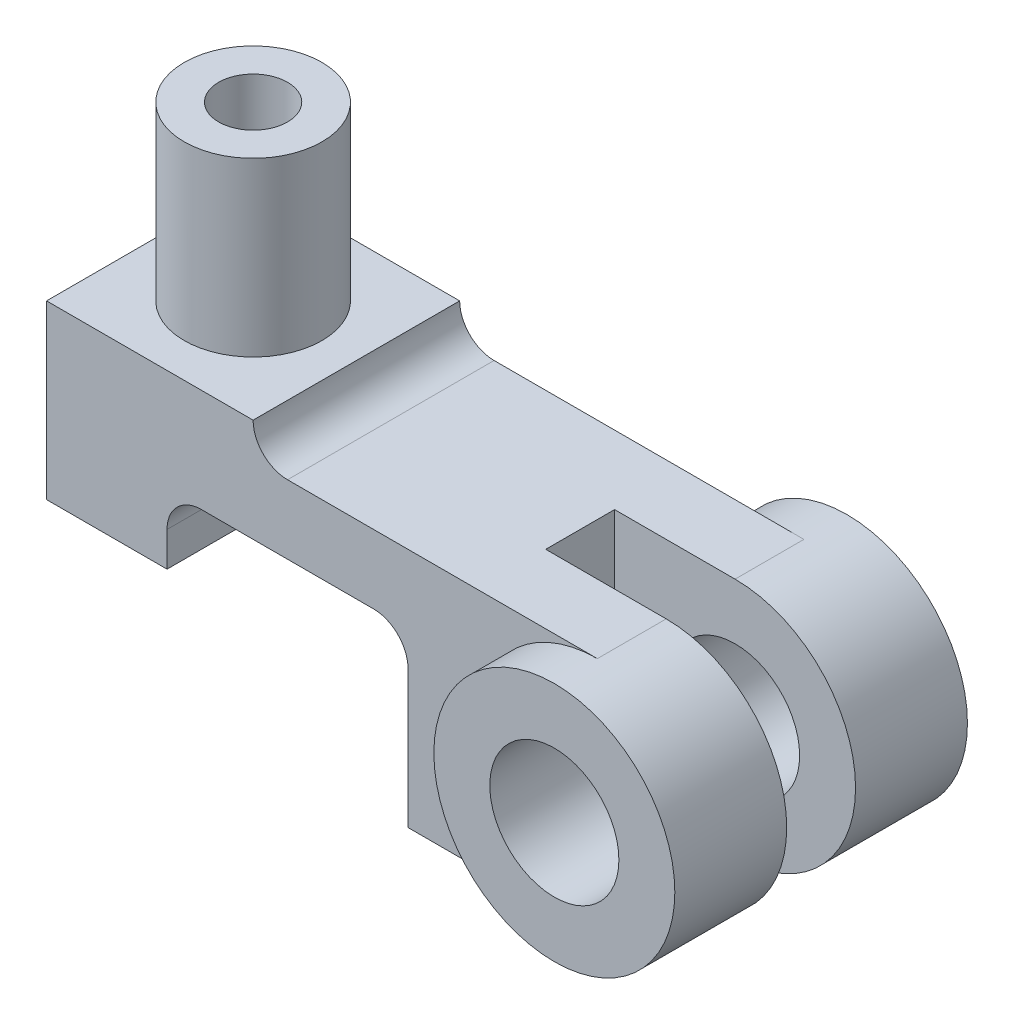
ISO-10303-21;
HEADER;
FILE_DESCRIPTION(('STEP AP214'),'2;1');
FILE_NAME('part.step','',(''),(''),'','','');
FILE_SCHEMA(('AUTOMOTIVE_DESIGN { 1 0 10303 214 1 1 1 1 }'));
ENDSEC;
DATA;
#1=APPLICATION_CONTEXT('core data for automotive mechanical design processes');
#2=APPLICATION_PROTOCOL_DEFINITION('international standard','automotive_design',2000,#1);
#3=PRODUCT_CONTEXT('',#1,'mechanical');
#4=PRODUCT('Part','Part','',(#3));
#5=PRODUCT_RELATED_PRODUCT_CATEGORY('part','',(#4));
#6=PRODUCT_DEFINITION_FORMATION('','',#4);
#7=PRODUCT_DEFINITION_CONTEXT('part definition',#1,'design');
#8=PRODUCT_DEFINITION('design','',#6,#7);
#9=PRODUCT_DEFINITION_SHAPE('','',#8);
#10=(LENGTH_UNIT() NAMED_UNIT(*) SI_UNIT(.MILLI.,.METRE.));
#11=(NAMED_UNIT(*) PLANE_ANGLE_UNIT() SI_UNIT($,.RADIAN.));
#12=(NAMED_UNIT(*) SI_UNIT($,.STERADIAN.) SOLID_ANGLE_UNIT());
#13=UNCERTAINTY_MEASURE_WITH_UNIT(LENGTH_MEASURE(1.E-05),#10,'distance_accuracy_value','');
#14=(GEOMETRIC_REPRESENTATION_CONTEXT(3) GLOBAL_UNCERTAINTY_ASSIGNED_CONTEXT((#13)) GLOBAL_UNIT_ASSIGNED_CONTEXT((#10,
#11,#12)) REPRESENTATION_CONTEXT('',''));
#15=CARTESIAN_POINT('',(0.,0.,0.));
#16=DIRECTION('',(0.,0.,1.));
#17=DIRECTION('',(1.,0.,0.));
#18=AXIS2_PLACEMENT_3D('',#15,#16,#17);
#19=CARTESIAN_POINT('',(128.,4.,34.));
#20=DIRECTION('',(0.,0.,-1.));
#21=DIRECTION('',(-1.,0.,0.));
#22=AXIS2_PLACEMENT_3D('',#19,#20,#21);
#23=CYLINDRICAL_SURFACE('',#22,28.);
#24=CARTESIAN_POINT('',(128.,4.,34.));
#25=DIRECTION('',(0.,0.,1.));
#26=DIRECTION('',(1.,0.,0.));
#27=AXIS2_PLACEMENT_3D('',#24,#25,#26);
#28=CIRCLE('',#27,28.);
#29=CARTESIAN_POINT('',(156.,4.,34.));
#30=VERTEX_POINT('',#29);
#31=EDGE_CURVE('E295',#30,#30,#28,.T.);
#32=ORIENTED_EDGE('',*,*,#31,.F.);
#33=EDGE_LOOP('',(#32));
#34=FACE_BOUND('',#33,.T.);
#35=CARTESIAN_POINT('',(128.,4.,8.));
#36=DIRECTION('',(0.,0.,1.));
#37=DIRECTION('',(1.,0.,0.));
#38=AXIS2_PLACEMENT_3D('',#35,#36,#37);
#39=CIRCLE('',#38,28.);
#40=CARTESIAN_POINT('',(128.,-24.,8.));
#41=VERTEX_POINT('',#40);
#42=CARTESIAN_POINT('',(128.,32.,8.));
#43=VERTEX_POINT('',#42);
#44=EDGE_CURVE('E11',#41,#43,#39,.T.);
#45=ORIENTED_EDGE('',*,*,#44,.T.);
#46=DIRECTION('',(0.,0.,-1.));
#47=VECTOR('',#46,1.);
#48=CARTESIAN_POINT('',(128.,32.,24.));
#49=LINE('',#48,#47);
#50=CARTESIAN_POINT('',(128.,32.,24.));
#51=VERTEX_POINT('',#50);
#52=EDGE_CURVE('E195',#51,#43,#49,.T.);
#53=ORIENTED_EDGE('',*,*,#52,.F.);
#54=CARTESIAN_POINT('',(128.,4.,24.));
#55=DIRECTION('',(0.,0.,-1.));
#56=DIRECTION('',(-1.,0.,0.));
#57=AXIS2_PLACEMENT_3D('',#54,#55,#56);
#58=CIRCLE('',#57,28.);
#59=CARTESIAN_POINT('',(128.,-24.,24.));
#60=VERTEX_POINT('',#59);
#61=EDGE_CURVE('E148',#51,#60,#58,.F.);
#62=ORIENTED_EDGE('',*,*,#61,.T.);
#63=DIRECTION('',(0.,0.,-1.));
#64=VECTOR('',#63,1.);
#65=CARTESIAN_POINT('',(128.,-24.,24.));
#66=LINE('',#65,#64);
#67=EDGE_CURVE('E197',#60,#41,#66,.T.);
#68=ORIENTED_EDGE('',*,*,#67,.T.);
#69=EDGE_LOOP('',(#45,#53,#62,#68));
#70=FACE_BOUND('',#69,.T.);
#71=ADVANCED_FACE('F39',(#34,#70),#23,.T.);
#72=CARTESIAN_POINT('',(0.,40.,24.));
#73=DIRECTION('',(1.,0.,0.));
#74=DIRECTION('',(0.,1.,0.));
#75=AXIS2_PLACEMENT_3D('',#72,#73,#74);
#76=PLANE('',#75);
#77=DIRECTION('',(0.,-1.,0.));
#78=VECTOR('',#77,1.);
#79=CARTESIAN_POINT('',(0.,40.,-24.));
#80=LINE('',#79,#78);
#81=CARTESIAN_POINT('',(0.,40.,-24.));
#82=VERTEX_POINT('',#81);
#83=CARTESIAN_POINT('',(0.,0.,-24.));
#84=VERTEX_POINT('',#83);
#85=EDGE_CURVE('E169',#82,#84,#80,.T.);
#86=ORIENTED_EDGE('',*,*,#85,.T.);
#87=DIRECTION('',(0.,0.,-1.));
#88=VECTOR('',#87,1.);
#89=CARTESIAN_POINT('',(0.,0.,24.));
#90=LINE('',#89,#88);
#91=CARTESIAN_POINT('',(0.,0.,24.));
#92=VERTEX_POINT('',#91);
#93=EDGE_CURVE('E217',#92,#84,#90,.T.);
#94=ORIENTED_EDGE('',*,*,#93,.F.);
#95=DIRECTION('',(0.,-1.,0.));
#96=VECTOR('',#95,1.);
#97=CARTESIAN_POINT('',(0.,40.,24.));
#98=LINE('',#97,#96);
#99=CARTESIAN_POINT('',(0.,40.,24.));
#100=VERTEX_POINT('',#99);
#101=EDGE_CURVE('E193',#100,#92,#98,.T.);
#102=ORIENTED_EDGE('',*,*,#101,.F.);
#103=DIRECTION('',(0.,0.,-1.));
#104=VECTOR('',#103,1.);
#105=CARTESIAN_POINT('',(0.,40.,24.));
#106=LINE('',#105,#104);
#107=EDGE_CURVE('E163',#100,#82,#106,.T.);
#108=ORIENTED_EDGE('',*,*,#107,.T.);
#109=EDGE_LOOP('',(#86,#94,#102,#108));
#110=FACE_BOUND('',#109,.T.);
#111=ADVANCED_FACE('F41',(#110),#76,.F.);
#112=CARTESIAN_POINT('',(0.,0.,24.));
#113=DIRECTION('',(0.,1.,0.));
#114=DIRECTION('',(0.,0.,1.));
#115=AXIS2_PLACEMENT_3D('',#112,#113,#114);
#116=PLANE('',#115);
#117=DIRECTION('',(1.,0.,0.));
#118=VECTOR('',#117,1.);
#119=CARTESIAN_POINT('',(0.,0.,-24.));
#120=LINE('',#119,#118);
#121=CARTESIAN_POINT('',(28.,0.,-24.));
#122=VERTEX_POINT('',#121);
#123=EDGE_CURVE('E173',#84,#122,#120,.T.);
#124=ORIENTED_EDGE('',*,*,#123,.T.);
#125=DIRECTION('',(0.,0.,-1.));
#126=VECTOR('',#125,1.);
#127=CARTESIAN_POINT('',(28.,0.,24.));
#128=LINE('',#127,#126);
#129=CARTESIAN_POINT('',(28.,0.,24.));
#130=VERTEX_POINT('',#129);
#131=EDGE_CURVE('E214',#130,#122,#128,.T.);
#132=ORIENTED_EDGE('',*,*,#131,.F.);
#133=DIRECTION('',(1.,0.,0.));
#134=VECTOR('',#133,1.);
#135=CARTESIAN_POINT('',(0.,0.,24.));
#136=LINE('',#135,#134);
#137=EDGE_CURVE('E113',#92,#130,#136,.T.);
#138=ORIENTED_EDGE('',*,*,#137,.F.);
#139=ORIENTED_EDGE('',*,*,#93,.T.);
#140=EDGE_LOOP('',(#124,#132,#138,#139));
#141=FACE_BOUND('',#140,.T.);
#142=ADVANCED_FACE('F348',(#141),#116,.F.);
#143=CARTESIAN_POINT('',(28.,0.,24.));
#144=DIRECTION('',(-1.,0.,0.));
#145=DIRECTION('',(0.,0.,1.));
#146=AXIS2_PLACEMENT_3D('',#143,#144,#145);
#147=PLANE('',#146);
#148=DIRECTION('',(0.,1.,0.));
#149=VECTOR('',#148,1.);
#150=CARTESIAN_POINT('',(28.,0.,-24.));
#151=LINE('',#150,#149);
#152=CARTESIAN_POINT('',(28.,7.99999999999994,-24.));
#153=VERTEX_POINT('',#152);
#154=EDGE_CURVE('E174',#122,#153,#151,.T.);
#155=ORIENTED_EDGE('',*,*,#154,.T.);
#156=DIRECTION('',(0.,0.,-1.));
#157=VECTOR('',#156,1.);
#158=CARTESIAN_POINT('',(28.,7.99999999999994,24.));
#159=LINE('',#158,#157);
#160=CARTESIAN_POINT('',(28.,7.99999999999994,24.));
#161=VERTEX_POINT('',#160);
#162=EDGE_CURVE('E215',#161,#153,#159,.T.);
#163=ORIENTED_EDGE('',*,*,#162,.F.);
#164=DIRECTION('',(0.,1.,0.));
#165=VECTOR('',#164,1.);
#166=CARTESIAN_POINT('',(28.,0.,24.));
#167=LINE('',#166,#165);
#168=EDGE_CURVE('E306',#130,#161,#167,.T.);
#169=ORIENTED_EDGE('',*,*,#168,.F.);
#170=ORIENTED_EDGE('',*,*,#131,.T.);
#171=EDGE_LOOP('',(#155,#163,#169,#170));
#172=FACE_BOUND('',#171,.T.);
#173=ADVANCED_FACE('F464',(#172),#147,.F.);
#174=CARTESIAN_POINT('',(36.,8.,24.));
#175=DIRECTION('',(0.,0.,-1.));
#176=DIRECTION('',(-1.,0.,0.));
#177=AXIS2_PLACEMENT_3D('',#174,#175,#176);
#178=CYLINDRICAL_SURFACE('',#177,8.);
#179=CARTESIAN_POINT('',(36.,8.,-24.));
#180=DIRECTION('',(0.,0.,-1.));
#181=DIRECTION('',(-1.,0.,0.));
#182=AXIS2_PLACEMENT_3D('',#179,#180,#181);
#183=CIRCLE('',#182,8.);
#184=CARTESIAN_POINT('',(36.0000000000001,16.,-24.));
#185=VERTEX_POINT('',#184);
#186=EDGE_CURVE('E178',#153,#185,#183,.T.);
#187=ORIENTED_EDGE('',*,*,#186,.T.);
#188=DIRECTION('',(0.,0.,-1.));
#189=VECTOR('',#188,1.);
#190=CARTESIAN_POINT('',(36.0000000000001,16.,24.));
#191=LINE('',#190,#189);
#192=CARTESIAN_POINT('',(36.0000000000001,16.,24.));
#193=VERTEX_POINT('',#192);
#194=EDGE_CURVE('E207',#193,#185,#191,.T.);
#195=ORIENTED_EDGE('',*,*,#194,.F.);
#196=CARTESIAN_POINT('',(36.,8.,24.));
#197=DIRECTION('',(0.,0.,-1.));
#198=DIRECTION('',(-1.,0.,0.));
#199=AXIS2_PLACEMENT_3D('',#196,#197,#198);
#200=CIRCLE('',#199,8.);
#201=EDGE_CURVE('E309',#161,#193,#200,.T.);
#202=ORIENTED_EDGE('',*,*,#201,.F.);
#203=ORIENTED_EDGE('',*,*,#162,.T.);
#204=EDGE_LOOP('',(#187,#195,#202,#203));
#205=FACE_BOUND('',#204,.T.);
#206=ADVANCED_FACE('F455',(#205),#178,.F.);
#207=CARTESIAN_POINT('',(36.0000000000001,16.,24.));
#208=DIRECTION('',(0.,1.,0.));
#209=DIRECTION('',(0.,0.,1.));
#210=AXIS2_PLACEMENT_3D('',#207,#208,#209);
#211=PLANE('',#210);
#212=DIRECTION('',(1.,0.,0.));
#213=VECTOR('',#212,1.);
#214=CARTESIAN_POINT('',(36.0000000000001,16.,-24.));
#215=LINE('',#214,#213);
#216=CARTESIAN_POINT('',(75.9999999999999,16.,-24.));
#217=VERTEX_POINT('',#216);
#218=EDGE_CURVE('E177',#185,#217,#215,.T.);
#219=ORIENTED_EDGE('',*,*,#218,.T.);
#220=DIRECTION('',(0.,0.,-1.));
#221=VECTOR('',#220,1.);
#222=CARTESIAN_POINT('',(75.9999999999999,16.,24.));
#223=LINE('',#222,#221);
#224=CARTESIAN_POINT('',(75.9999999999999,16.,24.));
#225=VERTEX_POINT('',#224);
#226=EDGE_CURVE('E206',#225,#217,#223,.T.);
#227=ORIENTED_EDGE('',*,*,#226,.F.);
#228=DIRECTION('',(1.,0.,0.));
#229=VECTOR('',#228,1.);
#230=CARTESIAN_POINT('',(36.0000000000001,16.,24.));
#231=LINE('',#230,#229);
#232=EDGE_CURVE('E315',#193,#225,#231,.T.);
#233=ORIENTED_EDGE('',*,*,#232,.F.);
#234=ORIENTED_EDGE('',*,*,#194,.T.);
#235=EDGE_LOOP('',(#219,#227,#233,#234));
#236=FACE_BOUND('',#235,.T.);
#237=ADVANCED_FACE('F441',(#236),#211,.F.);
#238=CARTESIAN_POINT('',(76.,8.,24.));
#239=DIRECTION('',(0.,0.,-1.));
#240=DIRECTION('',(-1.,0.,0.));
#241=AXIS2_PLACEMENT_3D('',#238,#239,#240);
#242=CYLINDRICAL_SURFACE('',#241,8.);
#243=CARTESIAN_POINT('',(76.,8.,-24.));
#244=DIRECTION('',(0.,0.,-1.));
#245=DIRECTION('',(-1.,0.,0.));
#246=AXIS2_PLACEMENT_3D('',#243,#244,#245);
#247=CIRCLE('',#246,8.);
#248=CARTESIAN_POINT('',(84.,7.99999999999995,-24.));
#249=VERTEX_POINT('',#248);
#250=EDGE_CURVE('E176',#217,#249,#247,.T.);
#251=ORIENTED_EDGE('',*,*,#250,.T.);
#252=DIRECTION('',(0.,0.,-1.));
#253=VECTOR('',#252,1.);
#254=CARTESIAN_POINT('',(84.,7.99999999999995,24.));
#255=LINE('',#254,#253);
#256=CARTESIAN_POINT('',(84.,7.99999999999995,24.));
#257=VERTEX_POINT('',#256);
#258=EDGE_CURVE('E201',#257,#249,#255,.T.);
#259=ORIENTED_EDGE('',*,*,#258,.F.);
#260=CARTESIAN_POINT('',(76.,8.,24.));
#261=DIRECTION('',(0.,0.,-1.));
#262=DIRECTION('',(-1.,0.,0.));
#263=AXIS2_PLACEMENT_3D('',#260,#261,#262);
#264=CIRCLE('',#263,8.);
#265=EDGE_CURVE('E314',#225,#257,#264,.T.);
#266=ORIENTED_EDGE('',*,*,#265,.F.);
#267=ORIENTED_EDGE('',*,*,#226,.T.);
#268=EDGE_LOOP('',(#251,#259,#266,#267));
#269=FACE_BOUND('',#268,.T.);
#270=ADVANCED_FACE('F432',(#269),#242,.F.);
#271=CARTESIAN_POINT('',(84.,7.99999999999994,24.));
#272=DIRECTION('',(1.,0.,0.));
#273=DIRECTION('',(0.,0.,-1.));
#274=AXIS2_PLACEMENT_3D('',#271,#272,#273);
#275=PLANE('',#274);
#276=DIRECTION('',(0.,-1.,0.));
#277=VECTOR('',#276,1.);
#278=CARTESIAN_POINT('',(84.,7.99999999999994,-24.));
#279=LINE('',#278,#277);
#280=CARTESIAN_POINT('',(84.,-24.,-24.));
#281=VERTEX_POINT('',#280);
#282=EDGE_CURVE('E185',#249,#281,#279,.T.);
#283=ORIENTED_EDGE('',*,*,#282,.T.);
#284=DIRECTION('',(0.,0.,-1.));
#285=VECTOR('',#284,1.);
#286=CARTESIAN_POINT('',(84.,-24.,24.));
#287=LINE('',#286,#285);
#288=CARTESIAN_POINT('',(84.,-24.,24.));
#289=VERTEX_POINT('',#288);
#290=EDGE_CURVE('E199',#289,#281,#287,.T.);
#291=ORIENTED_EDGE('',*,*,#290,.F.);
#292=DIRECTION('',(0.,-1.,0.));
#293=VECTOR('',#292,1.);
#294=CARTESIAN_POINT('',(84.,7.99999999999994,24.));
#295=LINE('',#294,#293);
#296=EDGE_CURVE('E316',#257,#289,#295,.T.);
#297=ORIENTED_EDGE('',*,*,#296,.F.);
#298=ORIENTED_EDGE('',*,*,#258,.T.);
#299=EDGE_LOOP('',(#283,#291,#297,#298));
#300=FACE_BOUND('',#299,.T.);
#301=ADVANCED_FACE('F426',(#300),#275,.F.);
#302=CARTESIAN_POINT('',(84.,-24.,24.));
#303=DIRECTION('',(0.,1.,0.));
#304=DIRECTION('',(0.,0.,1.));
#305=AXIS2_PLACEMENT_3D('',#302,#303,#304);
#306=PLANE('',#305);
#307=DIRECTION('',(0.,0.,1.));
#308=VECTOR('',#307,1.);
#309=CARTESIAN_POINT('',(100.,-24.,8.));
#310=LINE('',#309,#308);
#311=CARTESIAN_POINT('',(100.,-24.,-8.));
#312=VERTEX_POINT('',#311);
#313=CARTESIAN_POINT('',(100.,-24.,8.));
#314=VERTEX_POINT('',#313);
#315=EDGE_CURVE('E272',#312,#314,#310,.T.);
#316=ORIENTED_EDGE('',*,*,#315,.T.);
#317=DIRECTION('',(1.,0.,0.));
#318=VECTOR('',#317,1.);
#319=CARTESIAN_POINT('',(100.,-24.,8.));
#320=LINE('',#319,#318);
#321=EDGE_CURVE('E276',#314,#41,#320,.T.);
#322=ORIENTED_EDGE('',*,*,#321,.T.);
#323=ORIENTED_EDGE('',*,*,#67,.F.);
#324=DIRECTION('',(1.,0.,0.));
#325=VECTOR('',#324,1.);
#326=CARTESIAN_POINT('',(84.,-24.,24.));
#327=LINE('',#326,#325);
#328=EDGE_CURVE('E149',#289,#60,#327,.T.);
#329=ORIENTED_EDGE('',*,*,#328,.F.);
#330=ORIENTED_EDGE('',*,*,#290,.T.);
#331=DIRECTION('',(1.,0.,0.));
#332=VECTOR('',#331,1.);
#333=CARTESIAN_POINT('',(84.,-24.,-24.));
#334=LINE('',#333,#332);
#335=CARTESIAN_POINT('',(128.,-24.,-24.));
#336=VERTEX_POINT('',#335);
#337=EDGE_CURVE('E184',#281,#336,#334,.T.);
#338=ORIENTED_EDGE('',*,*,#337,.T.);
#339=CARTESIAN_POINT('',(128.,-24.,-7.99999999999999));
#340=VERTEX_POINT('',#339);
#341=EDGE_CURVE('E198',#340,#336,#66,.T.);
#342=ORIENTED_EDGE('',*,*,#341,.F.);
#343=DIRECTION('',(-1.,0.,0.));
#344=VECTOR('',#343,1.);
#345=CARTESIAN_POINT('',(100.,-24.,-8.));
#346=LINE('',#345,#344);
#347=EDGE_CURVE('E54',#340,#312,#346,.T.);
#348=ORIENTED_EDGE('',*,*,#347,.T.);
#349=EDGE_LOOP('',(#316,#322,#323,#329,#330,#338,#342,#348));
#350=FACE_BOUND('',#349,.T.);
#351=ADVANCED_FACE('F240',(#350),#306,.F.);
#352=CARTESIAN_POINT('',(128.,32.,24.));
#353=DIRECTION('',(0.,-1.,0.));
#354=DIRECTION('',(1.,0.,0.));
#355=AXIS2_PLACEMENT_3D('',#352,#353,#354);
#356=PLANE('',#355);
#357=ORIENTED_EDGE('',*,*,#52,.T.);
#358=DIRECTION('',(1.,0.,0.));
#359=VECTOR('',#358,1.);
#360=CARTESIAN_POINT('',(100.,32.,8.));
#361=LINE('',#360,#359);
#362=CARTESIAN_POINT('',(100.,32.,8.));
#363=VERTEX_POINT('',#362);
#364=EDGE_CURVE('E281',#363,#43,#361,.T.);
#365=ORIENTED_EDGE('',*,*,#364,.F.);
#366=DIRECTION('',(0.,0.,1.));
#367=VECTOR('',#366,1.);
#368=CARTESIAN_POINT('',(100.,32.,8.));
#369=LINE('',#368,#367);
#370=CARTESIAN_POINT('',(100.,32.,-8.));
#371=VERTEX_POINT('',#370);
#372=EDGE_CURVE('E287',#371,#363,#369,.T.);
#373=ORIENTED_EDGE('',*,*,#372,.F.);
#374=DIRECTION('',(-1.,0.,0.));
#375=VECTOR('',#374,1.);
#376=CARTESIAN_POINT('',(100.,32.,-8.));
#377=LINE('',#376,#375);
#378=CARTESIAN_POINT('',(128.,32.,-8.));
#379=VERTEX_POINT('',#378);
#380=EDGE_CURVE('E268',#379,#371,#377,.T.);
#381=ORIENTED_EDGE('',*,*,#380,.F.);
#382=CARTESIAN_POINT('',(128.,32.,-24.));
#383=VERTEX_POINT('',#382);
#384=EDGE_CURVE('E157',#379,#383,#49,.T.);
#385=ORIENTED_EDGE('',*,*,#384,.T.);
#386=DIRECTION('',(-1.,0.,0.));
#387=VECTOR('',#386,1.);
#388=CARTESIAN_POINT('',(128.,32.,-24.));
#389=LINE('',#388,#387);
#390=CARTESIAN_POINT('',(56.,32.,-24.));
#391=VERTEX_POINT('',#390);
#392=EDGE_CURVE('E156',#383,#391,#389,.T.);
#393=ORIENTED_EDGE('',*,*,#392,.T.);
#394=DIRECTION('',(0.,0.,-1.));
#395=VECTOR('',#394,1.);
#396=CARTESIAN_POINT('',(56.,32.,24.));
#397=LINE('',#396,#395);
#398=CARTESIAN_POINT('',(56.,32.,24.));
#399=VERTEX_POINT('',#398);
#400=EDGE_CURVE('E155',#399,#391,#397,.T.);
#401=ORIENTED_EDGE('',*,*,#400,.F.);
#402=DIRECTION('',(-1.,0.,0.));
#403=VECTOR('',#402,1.);
#404=CARTESIAN_POINT('',(128.,32.,24.));
#405=LINE('',#404,#403);
#406=EDGE_CURVE('E139',#51,#399,#405,.T.);
#407=ORIENTED_EDGE('',*,*,#406,.F.);
#408=EDGE_LOOP('',(#357,#365,#373,#381,#385,#393,#401,#407));
#409=FACE_BOUND('',#408,.T.);
#410=ADVANCED_FACE('F153',(#409),#356,.F.);
#411=CARTESIAN_POINT('',(56.,40.,24.));
#412=DIRECTION('',(0.,0.,-1.));
#413=DIRECTION('',(-1.,0.,0.));
#414=AXIS2_PLACEMENT_3D('',#411,#412,#413);
#415=CYLINDRICAL_SURFACE('',#414,8.);
#416=CARTESIAN_POINT('',(56.,40.,-24.));
#417=DIRECTION('',(0.,0.,-1.));
#418=DIRECTION('',(-1.,0.,0.));
#419=AXIS2_PLACEMENT_3D('',#416,#417,#418);
#420=CIRCLE('',#419,8.);
#421=CARTESIAN_POINT('',(48.,40.,-24.));
#422=VERTEX_POINT('',#421);
#423=EDGE_CURVE('E186',#391,#422,#420,.T.);
#424=ORIENTED_EDGE('',*,*,#423,.T.);
#425=DIRECTION('',(0.,0.,-1.));
#426=VECTOR('',#425,1.);
#427=CARTESIAN_POINT('',(48.,40.,24.));
#428=LINE('',#427,#426);
#429=CARTESIAN_POINT('',(48.,40.,24.));
#430=VERTEX_POINT('',#429);
#431=EDGE_CURVE('E159',#430,#422,#428,.T.);
#432=ORIENTED_EDGE('',*,*,#431,.F.);
#433=CARTESIAN_POINT('',(56.,40.,24.));
#434=DIRECTION('',(0.,0.,-1.));
#435=DIRECTION('',(-1.,0.,0.));
#436=AXIS2_PLACEMENT_3D('',#433,#434,#435);
#437=CIRCLE('',#436,8.);
#438=EDGE_CURVE('E143',#399,#430,#437,.T.);
#439=ORIENTED_EDGE('',*,*,#438,.F.);
#440=ORIENTED_EDGE('',*,*,#400,.T.);
#441=EDGE_LOOP('',(#424,#432,#439,#440));
#442=FACE_BOUND('',#441,.T.);
#443=ADVANCED_FACE('F165',(#442),#415,.F.);
#444=CARTESIAN_POINT('',(48.,40.,24.));
#445=DIRECTION('',(0.,-1.,0.));
#446=DIRECTION('',(1.,0.,0.));
#447=AXIS2_PLACEMENT_3D('',#444,#445,#446);
#448=PLANE('',#447);
#449=CARTESIAN_POINT('',(24.,40.,0.));
#450=DIRECTION('',(0.,-1.,0.));
#451=DIRECTION('',(1.,0.,0.));
#452=AXIS2_PLACEMENT_3D('',#449,#450,#451);
#453=CIRCLE('',#452,16.);
#454=CARTESIAN_POINT('',(40.,40.,0.));
#455=VERTEX_POINT('',#454);
#456=EDGE_CURVE('E219',#455,#455,#453,.F.);
#457=ORIENTED_EDGE('',*,*,#456,.F.);
#458=EDGE_LOOP('',(#457));
#459=FACE_BOUND('',#458,.T.);
#460=DIRECTION('',(-1.,0.,0.));
#461=VECTOR('',#460,1.);
#462=CARTESIAN_POINT('',(48.,40.,-24.));
#463=LINE('',#462,#461);
#464=EDGE_CURVE('E106',#422,#82,#463,.T.);
#465=ORIENTED_EDGE('',*,*,#464,.T.);
#466=ORIENTED_EDGE('',*,*,#107,.F.);
#467=DIRECTION('',(-1.,0.,0.));
#468=VECTOR('',#467,1.);
#469=CARTESIAN_POINT('',(48.,40.,24.));
#470=LINE('',#469,#468);
#471=EDGE_CURVE('E64',#430,#100,#470,.T.);
#472=ORIENTED_EDGE('',*,*,#471,.F.);
#473=ORIENTED_EDGE('',*,*,#431,.T.);
#474=EDGE_LOOP('',(#465,#466,#472,#473));
#475=FACE_BOUND('',#474,.T.);
#476=ADVANCED_FACE('F365',(#459,#475),#448,.F.);
#477=CARTESIAN_POINT('',(36.,8.,24.));
#478=DIRECTION('',(0.,0.,-1.));
#479=DIRECTION('',(-1.,0.,0.));
#480=AXIS2_PLACEMENT_3D('',#477,#478,#479);
#481=PLANE('',#480);
#482=ORIENTED_EDGE('',*,*,#61,.F.);
#483=ORIENTED_EDGE('',*,*,#406,.T.);
#484=ORIENTED_EDGE('',*,*,#438,.T.);
#485=ORIENTED_EDGE('',*,*,#471,.T.);
#486=ORIENTED_EDGE('',*,*,#101,.T.);
#487=ORIENTED_EDGE('',*,*,#137,.T.);
#488=ORIENTED_EDGE('',*,*,#168,.T.);
#489=ORIENTED_EDGE('',*,*,#201,.T.);
#490=ORIENTED_EDGE('',*,*,#232,.T.);
#491=ORIENTED_EDGE('',*,*,#265,.T.);
#492=ORIENTED_EDGE('',*,*,#296,.T.);
#493=ORIENTED_EDGE('',*,*,#328,.T.);
#494=EDGE_LOOP('',(#482,#483,#484,#485,#486,#487,#488,#489,#490,#491,#492,#493));
#495=FACE_BOUND('',#494,.T.);
#496=ADVANCED_FACE('F140',(#495),#481,.F.);
#497=CARTESIAN_POINT('',(36.,8.,-24.));
#498=DIRECTION('',(0.,0.,-1.));
#499=DIRECTION('',(-1.,0.,0.));
#500=AXIS2_PLACEMENT_3D('',#497,#498,#499);
#501=PLANE('',#500);
#502=ORIENTED_EDGE('',*,*,#392,.F.);
#503=CARTESIAN_POINT('',(128.,4.,-24.));
#504=DIRECTION('',(0.,0.,-1.));
#505=DIRECTION('',(-1.,0.,0.));
#506=AXIS2_PLACEMENT_3D('',#503,#504,#505);
#507=CIRCLE('',#506,28.);
#508=EDGE_CURVE('E224',#383,#336,#507,.F.);
#509=ORIENTED_EDGE('',*,*,#508,.T.);
#510=ORIENTED_EDGE('',*,*,#337,.F.);
#511=ORIENTED_EDGE('',*,*,#282,.F.);
#512=ORIENTED_EDGE('',*,*,#250,.F.);
#513=ORIENTED_EDGE('',*,*,#218,.F.);
#514=ORIENTED_EDGE('',*,*,#186,.F.);
#515=ORIENTED_EDGE('',*,*,#154,.F.);
#516=ORIENTED_EDGE('',*,*,#123,.F.);
#517=ORIENTED_EDGE('',*,*,#85,.F.);
#518=ORIENTED_EDGE('',*,*,#464,.F.);
#519=ORIENTED_EDGE('',*,*,#423,.F.);
#520=EDGE_LOOP('',(#502,#509,#510,#511,#512,#513,#514,#515,#516,#517,#518,#519));
#521=FACE_BOUND('',#520,.T.);
#522=ADVANCED_FACE('F244',(#521),#501,.T.);
#523=CARTESIAN_POINT('',(24.,80.,0.));
#524=DIRECTION('',(0.,1.,0.));
#525=DIRECTION('',(-1.,0.,0.));
#526=AXIS2_PLACEMENT_3D('',#523,#524,#525);
#527=PLANE('',#526);
#528=CARTESIAN_POINT('',(24.,80.,0.));
#529=DIRECTION('',(0.,1.,0.));
#530=DIRECTION('',(-1.,0.,0.));
#531=AXIS2_PLACEMENT_3D('',#528,#529,#530);
#532=CIRCLE('',#531,16.);
#533=CARTESIAN_POINT('',(7.99999999999998,80.,0.));
#534=VERTEX_POINT('',#533);
#535=EDGE_CURVE('E175',#534,#534,#532,.T.);
#536=ORIENTED_EDGE('',*,*,#535,.T.);
#537=EDGE_LOOP('',(#536));
#538=FACE_BOUND('',#537,.T.);
#539=CARTESIAN_POINT('',(24.,80.,0.));
#540=DIRECTION('',(0.,1.,0.));
#541=DIRECTION('',(-1.,0.,0.));
#542=AXIS2_PLACEMENT_3D('',#539,#540,#541);
#543=CIRCLE('',#542,8.);
#544=CARTESIAN_POINT('',(16.,80.,0.));
#545=VERTEX_POINT('',#544);
#546=EDGE_CURVE('E299',#545,#545,#543,.T.);
#547=ORIENTED_EDGE('',*,*,#546,.F.);
#548=EDGE_LOOP('',(#547));
#549=FACE_BOUND('',#548,.T.);
#550=ADVANCED_FACE('F382',(#538,#549),#527,.T.);
#551=CARTESIAN_POINT('',(24.,80.,0.));
#552=DIRECTION('',(0.,-1.,0.));
#553=DIRECTION('',(1.,0.,0.));
#554=AXIS2_PLACEMENT_3D('',#551,#552,#553);
#555=CYLINDRICAL_SURFACE('',#554,16.);
#556=ORIENTED_EDGE('',*,*,#535,.F.);
#557=EDGE_LOOP('',(#556));
#558=FACE_BOUND('',#557,.T.);
#559=ORIENTED_EDGE('',*,*,#456,.T.);
#560=EDGE_LOOP('',(#559));
#561=FACE_BOUND('',#560,.T.);
#562=ADVANCED_FACE('F369',(#558,#561),#555,.T.);
#563=CARTESIAN_POINT('',(24.,80.,0.));
#564=DIRECTION('',(0.,-1.,0.));
#565=DIRECTION('',(1.,0.,0.));
#566=AXIS2_PLACEMENT_3D('',#563,#564,#565);
#567=CYLINDRICAL_SURFACE('',#566,8.);
#568=ORIENTED_EDGE('',*,*,#546,.T.);
#569=EDGE_LOOP('',(#568));
#570=FACE_BOUND('',#569,.T.);
#571=CARTESIAN_POINT('',(24.,40.,0.));
#572=DIRECTION('',(0.,1.,0.));
#573=DIRECTION('',(-1.,0.,0.));
#574=AXIS2_PLACEMENT_3D('',#571,#572,#573);
#575=CIRCLE('',#574,8.);
#576=CARTESIAN_POINT('',(16.,40.,0.));
#577=VERTEX_POINT('',#576);
#578=EDGE_CURVE('E296',#577,#577,#575,.T.);
#579=ORIENTED_EDGE('',*,*,#578,.F.);
#580=EDGE_LOOP('',(#579));
#581=FACE_BOUND('',#580,.T.);
#582=ADVANCED_FACE('F363',(#570,#581),#567,.F.);
#583=ORIENTED_EDGE('',*,*,#578,.T.);
#584=EDGE_LOOP('',(#583));
#585=FACE_BOUND('',#584,.T.);
#586=ADVANCED_FACE('F352',(#585),#448,.F.);
#587=ORIENTED_EDGE('',*,*,#384,.F.);
#588=CARTESIAN_POINT('',(128.,4.,-8.));
#589=DIRECTION('',(0.,0.,-1.));
#590=DIRECTION('',(-1.,0.,0.));
#591=AXIS2_PLACEMENT_3D('',#588,#589,#590);
#592=CIRCLE('',#591,28.);
#593=EDGE_CURVE('E48',#379,#340,#592,.T.);
#594=ORIENTED_EDGE('',*,*,#593,.T.);
#595=ORIENTED_EDGE('',*,*,#341,.T.);
#596=ORIENTED_EDGE('',*,*,#508,.F.);
#597=EDGE_LOOP('',(#587,#594,#595,#596));
#598=FACE_BOUND('',#597,.T.);
#599=CARTESIAN_POINT('',(128.,4.,-34.));
#600=DIRECTION('',(0.,0.,1.));
#601=DIRECTION('',(1.,0.,0.));
#602=AXIS2_PLACEMENT_3D('',#599,#600,#601);
#603=CIRCLE('',#602,28.);
#604=CARTESIAN_POINT('',(156.,4.,-34.));
#605=VERTEX_POINT('',#604);
#606=EDGE_CURVE('E286',#605,#605,#603,.T.);
#607=ORIENTED_EDGE('',*,*,#606,.T.);
#608=EDGE_LOOP('',(#607));
#609=FACE_BOUND('',#608,.T.);
#610=ADVANCED_FACE('F229',(#598,#609),#23,.T.);
#611=CARTESIAN_POINT('',(128.,4.,34.));
#612=DIRECTION('',(0.,0.,1.));
#613=DIRECTION('',(1.,0.,0.));
#614=AXIS2_PLACEMENT_3D('',#611,#612,#613);
#615=PLANE('',#614);
#616=CARTESIAN_POINT('',(128.,4.,34.));
#617=DIRECTION('',(0.,0.,1.));
#618=DIRECTION('',(1.,0.,0.));
#619=AXIS2_PLACEMENT_3D('',#616,#617,#618);
#620=CIRCLE('',#619,15.);
#621=CARTESIAN_POINT('',(143.,4.,34.));
#622=VERTEX_POINT('',#621);
#623=EDGE_CURVE('E328',#622,#622,#620,.T.);
#624=ORIENTED_EDGE('',*,*,#623,.F.);
#625=EDGE_LOOP('',(#624));
#626=FACE_BOUND('',#625,.T.);
#627=ORIENTED_EDGE('',*,*,#31,.T.);
#628=EDGE_LOOP('',(#627));
#629=FACE_BOUND('',#628,.T.);
#630=ADVANCED_FACE('F338',(#626,#629),#615,.T.);
#631=CARTESIAN_POINT('',(128.,4.,-34.));
#632=DIRECTION('',(0.,0.,1.));
#633=DIRECTION('',(1.,0.,0.));
#634=AXIS2_PLACEMENT_3D('',#631,#632,#633);
#635=PLANE('',#634);
#636=CARTESIAN_POINT('',(128.,4.,-34.));
#637=DIRECTION('',(0.,0.,1.));
#638=DIRECTION('',(1.,0.,0.));
#639=AXIS2_PLACEMENT_3D('',#636,#637,#638);
#640=CIRCLE('',#639,15.);
#641=CARTESIAN_POINT('',(143.,4.,-34.));
#642=VERTEX_POINT('',#641);
#643=EDGE_CURVE('E326',#642,#642,#640,.T.);
#644=ORIENTED_EDGE('',*,*,#643,.T.);
#645=EDGE_LOOP('',(#644));
#646=FACE_BOUND('',#645,.T.);
#647=ORIENTED_EDGE('',*,*,#606,.F.);
#648=EDGE_LOOP('',(#647));
#649=FACE_BOUND('',#648,.T.);
#650=ADVANCED_FACE('F339',(#646,#649),#635,.F.);
#651=CARTESIAN_POINT('',(100.,-24.,8.));
#652=DIRECTION('',(0.,0.,1.));
#653=DIRECTION('',(1.,0.,0.));
#654=AXIS2_PLACEMENT_3D('',#651,#652,#653);
#655=PLANE('',#654);
#656=CARTESIAN_POINT('',(128.,4.,8.));
#657=DIRECTION('',(0.,0.,1.));
#658=DIRECTION('',(1.,0.,0.));
#659=AXIS2_PLACEMENT_3D('',#656,#657,#658);
#660=CIRCLE('',#659,15.);
#661=CARTESIAN_POINT('',(143.,4.,7.99999999999999));
#662=VERTEX_POINT('',#661);
#663=EDGE_CURVE('E288',#662,#662,#660,.T.);
#664=ORIENTED_EDGE('',*,*,#663,.T.);
#665=EDGE_LOOP('',(#664));
#666=FACE_BOUND('',#665,.T.);
#667=ORIENTED_EDGE('',*,*,#44,.F.);
#668=ORIENTED_EDGE('',*,*,#321,.F.);
#669=DIRECTION('',(0.,1.,0.));
#670=VECTOR('',#669,1.);
#671=CARTESIAN_POINT('',(100.,-24.,8.));
#672=LINE('',#671,#670);
#673=EDGE_CURVE('E275',#314,#363,#672,.T.);
#674=ORIENTED_EDGE('',*,*,#673,.T.);
#675=ORIENTED_EDGE('',*,*,#364,.T.);
#676=EDGE_LOOP('',(#667,#668,#674,#675));
#677=FACE_BOUND('',#676,.T.);
#678=ADVANCED_FACE('F325',(#666,#677),#655,.F.);
#679=CARTESIAN_POINT('',(100.,-24.,-8.));
#680=DIRECTION('',(0.,0.,-1.));
#681=DIRECTION('',(-1.,0.,0.));
#682=AXIS2_PLACEMENT_3D('',#679,#680,#681);
#683=PLANE('',#682);
#684=CARTESIAN_POINT('',(128.,4.,-8.));
#685=DIRECTION('',(0.,0.,-1.));
#686=DIRECTION('',(-1.,0.,0.));
#687=AXIS2_PLACEMENT_3D('',#684,#685,#686);
#688=CIRCLE('',#687,15.);
#689=CARTESIAN_POINT('',(113.,4.,-8.));
#690=VERTEX_POINT('',#689);
#691=EDGE_CURVE('E43',#690,#690,#688,.T.);
#692=ORIENTED_EDGE('',*,*,#691,.T.);
#693=EDGE_LOOP('',(#692));
#694=FACE_BOUND('',#693,.T.);
#695=ORIENTED_EDGE('',*,*,#380,.T.);
#696=DIRECTION('',(0.,1.,0.));
#697=VECTOR('',#696,1.);
#698=CARTESIAN_POINT('',(100.,-24.,-8.));
#699=LINE('',#698,#697);
#700=EDGE_CURVE('E264',#312,#371,#699,.T.);
#701=ORIENTED_EDGE('',*,*,#700,.F.);
#702=ORIENTED_EDGE('',*,*,#347,.F.);
#703=ORIENTED_EDGE('',*,*,#593,.F.);
#704=EDGE_LOOP('',(#695,#701,#702,#703));
#705=FACE_BOUND('',#704,.T.);
#706=ADVANCED_FACE('F270',(#694,#705),#683,.F.);
#707=CARTESIAN_POINT('',(100.,-24.,8.));
#708=DIRECTION('',(-1.,0.,0.));
#709=DIRECTION('',(0.,-1.,0.));
#710=AXIS2_PLACEMENT_3D('',#707,#708,#709);
#711=PLANE('',#710);
#712=ORIENTED_EDGE('',*,*,#372,.T.);
#713=ORIENTED_EDGE('',*,*,#673,.F.);
#714=ORIENTED_EDGE('',*,*,#315,.F.);
#715=ORIENTED_EDGE('',*,*,#700,.T.);
#716=EDGE_LOOP('',(#712,#713,#714,#715));
#717=FACE_BOUND('',#716,.T.);
#718=ADVANCED_FACE('F274',(#717),#711,.F.);
#719=CARTESIAN_POINT('',(128.,4.,34.));
#720=DIRECTION('',(0.,0.,1.));
#721=DIRECTION('',(1.,0.,0.));
#722=AXIS2_PLACEMENT_3D('',#719,#720,#721);
#723=CYLINDRICAL_SURFACE('',#722,15.);
#724=ORIENTED_EDGE('',*,*,#643,.F.);
#725=EDGE_LOOP('',(#724));
#726=FACE_BOUND('',#725,.T.);
#727=ORIENTED_EDGE('',*,*,#691,.F.);
#728=EDGE_LOOP('',(#727));
#729=FACE_BOUND('',#728,.T.);
#730=ADVANCED_FACE('F564',(#726,#729),#723,.F.);
#731=ORIENTED_EDGE('',*,*,#623,.T.);
#732=EDGE_LOOP('',(#731));
#733=FACE_BOUND('',#732,.T.);
#734=ORIENTED_EDGE('',*,*,#663,.F.);
#735=EDGE_LOOP('',(#734));
#736=FACE_BOUND('',#735,.T.);
#737=ADVANCED_FACE('F334',(#733,#736),#723,.F.);
#738=CLOSED_SHELL('',(#71,#111,#142,#173,#206,#237,#270,#301,#351,#410,#443,#476,#496,#522,#550,
#562,#582,#586,#610,#630,#650,#678,#706,#718,#730,#737));
#739=MANIFOLD_SOLID_BREP('B2',#738);
#740=ADVANCED_BREP_SHAPE_REPRESENTATION('',(#18,#739),#14);
#741=SHAPE_DEFINITION_REPRESENTATION(#9,#740);
ENDSEC;
END-ISO-10303-21;
